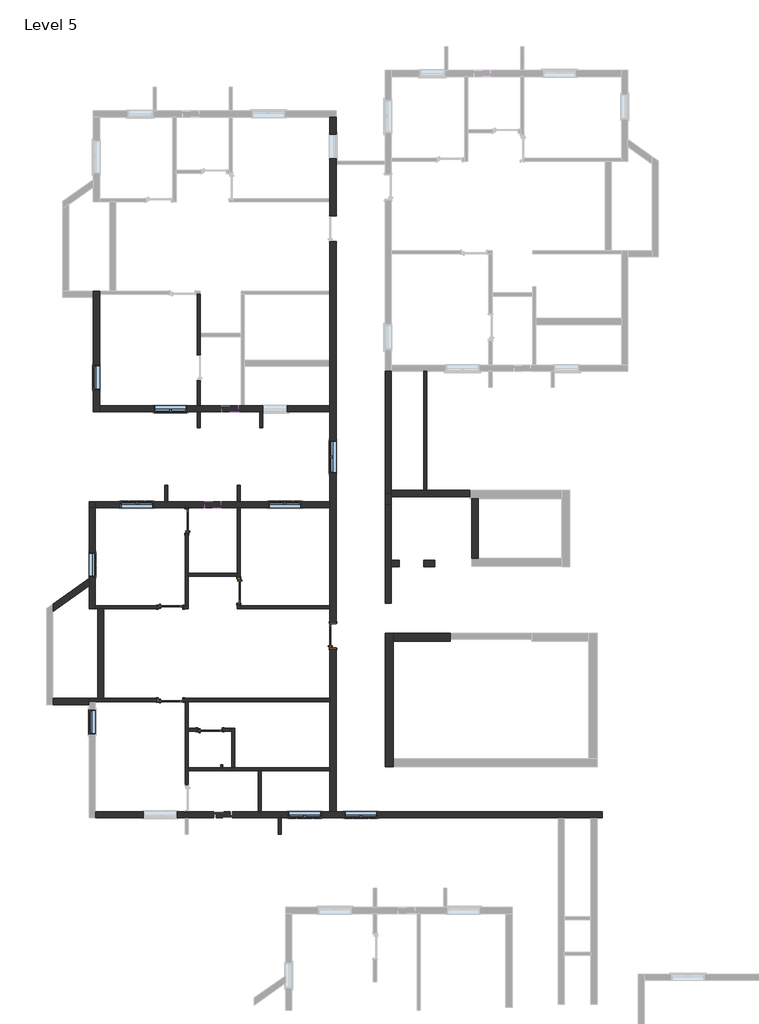
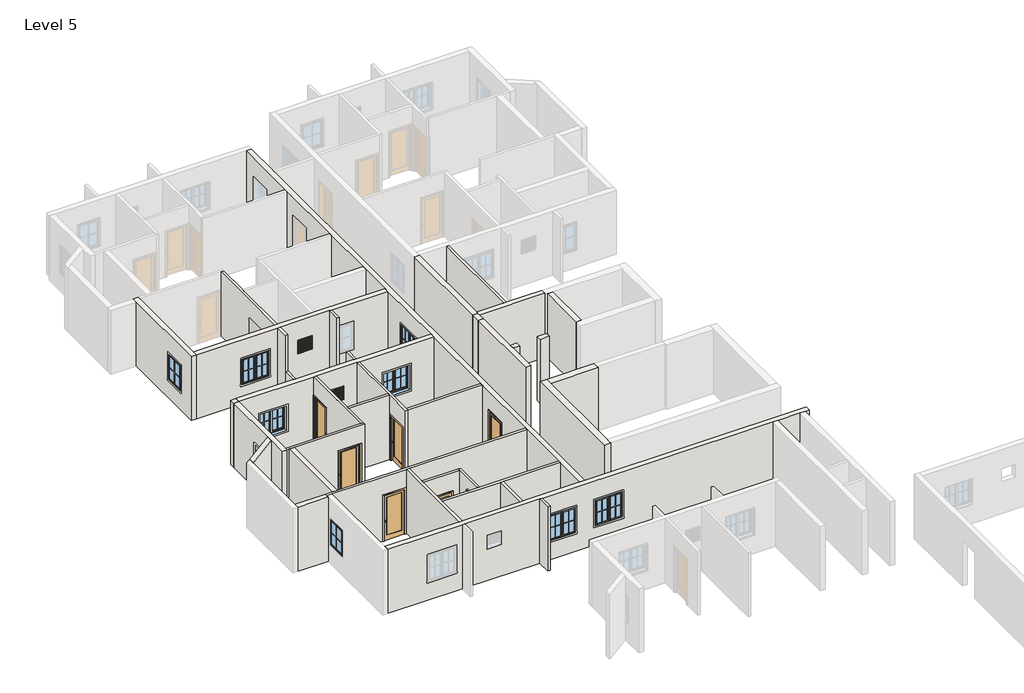
# One storey, part 4 of 7: 38 walls, 11 windows, 6 doors.
"""IFC4 building model written with IfcOpenShell, lengths in millimetres."""

from ifc_helpers import new_model, si_unit, frame, origin, place, context, project, spatial, polyline, outline, extrude, faceted_brep, transform, mapped, element, save
from components import door_a3feeac7, door_3c6ab76a, door_3b97b8e7, window_272f20d6, window_casement_double_4_x_4_af3140d2, window_f2d8fef0

model = new_model("IFC4")

# Units and contexts
model_context = context("Model", 3, world=origin())
ifc_project = project(units=[si_unit("LENGTHUNIT", "METRE", prefix="MILLI")], contexts=[model_context])

# Site, building, storey
site = spatial("IfcSite", under=ifc_project)
building = spatial("IfcBuilding", under=site)
storey = spatial("IfcBuildingStorey", under=building, Name="Level 5", Elevation=6400.8)

# Doors
placement = place(None, origin())
door_shape = door_a3feeac7(model_context)
element("IfcDoor", 1, ObjectType="Door-Interior-Single-1_Panel-Wood : 2'6\" x 7' door", at=placement, inside=storey, context=model_context, shape_type="MappedRepresentation", body=[
    mapped(door_shape, transform((-11252.4759469, 12427.2461172, 6400.8), x_axis=(0.0, 1.0, 0.0), y_axis=(-1.0, 0.0, 0.0), z_axis=(0.0, 0.0, 1.0))),
])
element("IfcDoor", 2, ObjectType="Door-Interior-Single-1_Panel-Wood : 2'6\" x 7' door", at=placement, inside=storey, context=model_context, shape_type="MappedRepresentation", body=[
    mapped(door_shape, transform((-10385.7009469, 4632.6211172, 6400.8), x_axis=(1.0, 0.0, 0.0), y_axis=(0.0, 1.0, 0.0), z_axis=(0.0, 0.0, 1.0))),
])
door_2_shape = door_3c6ab76a(model_context)
element("IfcDoor", 3, ObjectType="Door-Interior-Single-1_Panel-Wood : 36\" x 84\"", at=placement, inside=storey, context=model_context, shape_type="MappedRepresentation", body=[
    mapped(door_2_shape, transform((-9309.3759469, 9817.3961172, 6400.8), x_axis=(0.0, -1.0, 0.0), y_axis=(1.0, 0.0, 0.0), z_axis=(0.0, 0.0, 1.0))),
])
element("IfcDoor", 4, ObjectType="Door-Interior-Single-1_Panel-Wood : 36\" x 84\"", at=placement, inside=storey, context=model_context, shape_type="MappedRepresentation", body=[
    mapped(door_2_shape, transform((-11865.2509469, 9210.9711172, 6400.8), x_axis=(1.0, 0.0, 0.0), y_axis=(0.0, 1.0, 0.0), z_axis=(0.0, 0.0, 1.0))),
])
door_3_shape = door_3b97b8e7(model_context)
element("IfcDoor", 5, ObjectType="Door-Interior-Single-1_Panel-Wood : 36\" x 84\"", at=placement, inside=storey, context=model_context, shape_type="MappedRepresentation", body=[
    mapped(door_3_shape, transform((-5791.4759469, 8140.9961172, 6400.8), x_axis=(0.0, 1.0, 0.0), y_axis=(-1.0, 0.0, 0.0), z_axis=(0.0, 0.0, 1.0))),
])
element("IfcDoor", 6, ObjectType="Door-Interior-Single-1_Panel-Wood : 36\" x 84\"", at=placement, inside=storey, context=model_context, shape_type="MappedRepresentation", body=[
    mapped(door_shape, transform((-11865.2509469, 5737.5211172, 6400.8), x_axis=(1.0, 0.0, 0.0), y_axis=(0.0, 1.0, 0.0), z_axis=(0.0, 0.0, 1.0))),
])

# Walls
element("IfcWall", 7, ObjectType="1' feet", at=placement, inside=storey, context=model_context, shape_type="Brep", body=[
    faceted_brep([(-3540.4009469, 3245.1461172, 6400.8), (-3540.4009469, 3549.9461172, 6400.8), (-3540.4009469, 7931.4461172, 6400.8), (-3540.4009469, 8236.2461172, 6400.8), (-3540.4009469, 8236.2461172, 9448.8), (-3540.4009469, 7931.4461172, 9448.8), (-3540.4009469, 3549.9461172, 9448.8), (-3540.4009469, 3245.1461172, 9448.8), (-3845.2009469, 3245.1461172, 6400.8), (-3845.2009469, 3245.1461172, 9448.8), (-3845.2009469, 8236.2461172, 9448.8), (-3845.2009469, 8236.2461172, 6400.8)], [[[0, 1, 2, 3, 4, 5, 6, 7]], [[8, 9, 10, 11]], [[3, 2, 1, 0, 8, 11]], [[7, 6, 5, 4, 10, 9]], [[4, 3, 11, 10]], [[0, 7, 9, 8]]]),
])
element("IfcWall", 8, ObjectType="1' feet", at=placement, inside=storey, context=model_context, shape_type="Brep", body=[
    faceted_brep([(-3540.4009469, 7931.4461172, 6400.8), (-1406.8009469, 7931.4461172, 6400.8), (-1406.8009469, 7931.4461172, 9448.8), (-3540.4009469, 7931.4461172, 9448.8), (-3540.4009469, 8236.2461172, 6400.8), (-3540.4009469, 8236.2461172, 9448.8), (-1406.8009469, 8236.2461172, 9448.8), (-1406.8009469, 8236.2461172, 6400.8), (-1406.8009469, 8007.6461172, 6400.8), (-1406.8009469, 8007.6461172, 9448.8)], [[[0, 1, 2, 3]], [[4, 5, 6, 7]], [[1, 0, 4, 7, 8]], [[2, 1, 8, 7, 6, 9]], [[3, 2, 9, 6, 5]], [[0, 3, 5, 4]]]),
])
element("IfcWall", 9, ObjectType="4.5\" wall", at=placement, inside=storey, context=model_context, shape_type="Brep", body=[
    faceted_brep([(-10741.3009469, 20898.1461172, 9448.8), (-10741.3009469, 19437.6461172, 9448.8), (-10741.3009469, 19323.3461172, 9448.8), (-10741.3009469, 16732.5461172, 9448.8), (-10741.3009469, 16732.5461172, 6400.8), (-10741.3009469, 17678.6961172, 6400.8), (-10741.3009469, 17678.6961172, 8559.8), (-10741.3009469, 18643.8961172, 8559.8), (-10741.3009469, 18643.8961172, 6400.8), (-10741.3009469, 19323.3461172, 6400.8), (-10741.3009469, 19437.6461172, 6400.8), (-10741.3009469, 20898.1461172, 6400.8), (-10855.6009469, 16732.5461172, 9448.8), (-10855.6009469, 20898.1461172, 9448.8), (-10855.6009469, 20898.1461172, 6400.8), (-10855.6009469, 18643.8961172, 6400.8), (-10855.6009469, 18643.8961172, 8559.8), (-10855.6009469, 17678.6961172, 8559.8), (-10855.6009469, 17678.6961172, 6400.8), (-10855.6009469, 16732.5461172, 6400.8)], [[[0, 1, 2, 3, 4, 5, 6, 7, 8, 9, 10, 11]], [[12, 13, 14, 15, 16, 17, 18, 19]], [[4, 19, 18, 5]], [[14, 11, 10, 9, 8, 15]], [[3, 2, 1, 0, 13, 12]], [[4, 3, 12, 19]], [[0, 11, 14, 13]], [[7, 16, 15, 8]], [[16, 7, 6, 17]], [[17, 6, 5, 18]]]),
])
element("IfcWall", 10, ObjectType="4.5\" wall", at=placement, inside=storey, context=model_context, shape_type="Brep", body=[
    faceted_brep([(-9369.7009469, 9150.6461172, 9448.8), (-9369.7009469, 10369.8461172, 9448.8), (-9369.7009469, 10484.1461172, 9448.8), (-9369.7009469, 12922.5461172, 9448.8), (-9369.7009469, 12922.5461172, 6400.8), (-9369.7009469, 10484.1461172, 6400.8), (-9369.7009469, 10369.8461172, 6400.8), (-9369.7009469, 10299.9961172, 6400.8), (-9369.7009469, 10299.9961172, 8559.8), (-9369.7009469, 9334.7961172, 8559.8), (-9369.7009469, 9334.7961172, 6400.8), (-9369.7009469, 9150.6461172, 6400.8), (-9255.4009469, 12922.5461172, 9448.8), (-9255.4009469, 9264.9461172, 9448.8), (-9255.4009469, 9150.6461172, 9448.8), (-9255.4009469, 9150.6461172, 6400.8), (-9255.4009469, 9264.9461172, 6400.8), (-9255.4009469, 9334.7961172, 6400.8), (-9255.4009469, 9334.7961172, 8559.8), (-9255.4009469, 10299.9961172, 8559.8), (-9255.4009469, 10299.9961172, 6400.8), (-9255.4009469, 12922.5461172, 6400.8)], [[[0, 1, 2, 3, 4, 5, 6, 7, 8, 9, 10, 11]], [[12, 13, 14, 15, 16, 17, 18, 19, 20, 21]], [[4, 21, 20, 7, 6, 5]], [[15, 11, 10, 17, 16]], [[3, 2, 1, 0, 14, 13, 12]], [[4, 3, 12, 21]], [[0, 11, 15, 14]], [[9, 18, 17, 10]], [[18, 9, 8, 19]], [[19, 8, 7, 20]]]),
])
element("IfcWall", 11, ObjectType="4.5\" wall", at=placement, inside=storey, context=model_context, shape_type="SweptSolid", body=[
    extrude(outline(polyline([(-11198.5009469, 10484.1461172), (-9369.7009469, 10484.1461172), (-9369.7009469, 10369.8461172), (-11198.5009469, 10369.8461172), (-11198.5009469, 10484.1461172)])), frame((0.0, 0.0, 6400.8), z_axis=(0.0, 0.0, 1.0), x_axis=(1.0, 0.0, 0.0)), (0.0, 0.0, 1.0), 3048.0),
])
element("IfcWall", 12, ObjectType="4.5\" wall", at=placement, inside=storey, context=model_context, shape_type="Brep", body=[
    faceted_brep([(-11312.8009469, 9264.9461172, 9448.8), (-11312.8009469, 12922.5461172, 9448.8), (-11312.8009469, 12922.5461172, 6400.8), (-11312.8009469, 12909.8461172, 6400.8), (-11312.8009469, 12909.8461172, 8559.8), (-11312.8009469, 11944.6461172, 8559.8), (-11312.8009469, 11944.6461172, 6400.8), (-11312.8009469, 9264.9461172, 6400.8), (-11198.5009469, 12922.5461172, 9448.8), (-11198.5009469, 10484.1461172, 9448.8), (-11198.5009469, 10369.8461172, 9448.8), (-11198.5009469, 9264.9461172, 9448.8), (-11198.5009469, 9264.9461172, 6400.8), (-11198.5009469, 10369.8461172, 6400.8), (-11198.5009469, 10484.1461172, 6400.8), (-11198.5009469, 11944.6461172, 6400.8), (-11198.5009469, 11944.6461172, 8559.8), (-11198.5009469, 12909.8461172, 8559.8), (-11198.5009469, 12909.8461172, 6400.8), (-11198.5009469, 12922.5461172, 6400.8)], [[[0, 1, 2, 3, 4, 5, 6, 7]], [[8, 9, 10, 11, 12, 13, 14, 15, 16, 17, 18, 19]], [[12, 7, 6, 15, 14, 13]], [[2, 19, 18, 3]], [[1, 0, 11, 10, 9, 8]], [[0, 7, 12, 11]], [[2, 1, 8, 19]], [[17, 4, 3, 18]], [[4, 17, 16, 5]], [[5, 16, 15, 6]]]),
])
element("IfcWall", 13, ObjectType="4.5\" wall", at=placement, inside=storey, context=model_context, shape_type="Brep", body=[
    faceted_brep([(-14665.6009469, 9264.9461172, 9448.8), (-11312.8009469, 9264.9461172, 9448.8), (-11198.5009469, 9264.9461172, 9448.8), (-11198.5009469, 9264.9461172, 6400.8), (-11312.8009469, 9264.9461172, 6400.8), (-11382.6509469, 9264.9461172, 6400.8), (-11382.6509469, 9264.9461172, 8559.8), (-12347.8509469, 9264.9461172, 8559.8), (-12347.8509469, 9264.9461172, 6400.8), (-14665.6009469, 9264.9461172, 6400.8), (-11198.5009469, 9150.6461172, 9448.8), (-14360.8009469, 9150.6461172, 9448.8), (-14589.4009469, 9150.6461172, 9448.8), (-14665.6009469, 9150.6461172, 9448.8), (-14665.6009469, 9150.6461172, 6400.8), (-14589.4009469, 9150.6461172, 6400.8), (-14360.8009469, 9150.6461172, 6400.8), (-12347.8509469, 9150.6461172, 6400.8), (-12347.8509469, 9150.6461172, 8559.8), (-11382.6509469, 9150.6461172, 8559.8), (-11382.6509469, 9150.6461172, 6400.8), (-11198.5009469, 9150.6461172, 6400.8)], [[[0, 1, 2, 3, 4, 5, 6, 7, 8, 9]], [[10, 11, 12, 13, 14, 15, 16, 17, 18, 19, 20, 21]], [[3, 21, 20, 5, 4]], [[14, 9, 8, 17, 16, 15]], [[2, 1, 0, 13, 12, 11, 10]], [[3, 2, 10, 21]], [[0, 9, 14, 13]], [[19, 6, 5, 20]], [[6, 19, 18, 7]], [[7, 18, 17, 8]]]),
])
element("IfcWall", 14, ObjectType="4.5\" wall", at=placement, inside=storey, context=model_context, shape_type="SweptSolid", body=[
    extrude(outline(polyline([(-9255.4009469, 9264.9461172), (-5902.6009469, 9264.9461172), (-5902.6009469, 9150.6461172), (-9255.4009469, 9150.6461172), (-9255.4009469, 9264.9461172)])), frame((0.0, 0.0, 6400.8), z_axis=(0.0, 0.0, 1.0), x_axis=(1.0, 0.0, 0.0)), (0.0, 0.0, 1.0), 3048.0),
])
element("IfcWall", 15, ObjectType="4.5\" wall", at=placement, inside=storey, context=model_context, shape_type="Brep", body=[
    faceted_brep([(-5902.6009469, 5683.5461172, 9448.8), (-11198.5009469, 5683.5461172, 9448.8), (-11312.8009469, 5683.5461172, 9448.8), (-14665.6009469, 5683.5461172, 9448.8), (-14894.2009469, 5683.5461172, 9448.8), (-14894.2009469, 5683.5461172, 6400.8), (-14665.6009469, 5683.5461172, 6400.8), (-12347.8509469, 5683.5461172, 6400.8), (-12347.8509469, 5683.5461172, 8559.8), (-11382.6509469, 5683.5461172, 8559.8), (-11382.6509469, 5683.5461172, 6400.8), (-11312.8009469, 5683.5461172, 6400.8), (-11198.5009469, 5683.5461172, 6400.8), (-5902.6009469, 5683.5461172, 6400.8), (-14894.2009469, 5797.8461172, 9448.8), (-14589.4009469, 5797.8461172, 9448.8), (-14360.8009469, 5797.8461172, 9448.8), (-5902.6009469, 5797.8461172, 9448.8), (-5902.6009469, 5797.8461172, 6400.8), (-11382.6509469, 5797.8461172, 6400.8), (-11382.6509469, 5797.8461172, 8559.8), (-12347.8509469, 5797.8461172, 8559.8), (-12347.8509469, 5797.8461172, 6400.8), (-14360.8009469, 5797.8461172, 6400.8), (-14589.4009469, 5797.8461172, 6400.8), (-14894.2009469, 5797.8461172, 6400.8)], [[[0, 1, 2, 3, 4, 5, 6, 7, 8, 9, 10, 11, 12, 13]], [[14, 15, 16, 17, 18, 19, 20, 21, 22, 23, 24, 25]], [[18, 13, 12, 11, 10, 19]], [[5, 25, 24, 23, 22, 7, 6]], [[4, 3, 2, 1, 0, 17, 16, 15, 14]], [[0, 13, 18, 17]], [[5, 4, 14, 25]], [[9, 20, 19, 10]], [[20, 9, 8, 21]], [[21, 8, 7, 22]]]),
])
element("IfcWall", 16, ObjectType="4.5\" wall", at=placement, inside=storey, context=model_context, shape_type="Brep", body=[
    faceted_brep([(-11198.5009469, 5683.5461172, 9448.8), (-11198.5009469, 4692.9461172, 9448.8), (-11198.5009469, 4578.6461172, 9448.8), (-11198.5009469, 3207.0461172, 9448.8), (-11198.5009469, 3092.7461172, 9448.8), (-11198.5009469, 1568.7461172, 9448.8), (-11198.5009469, 1568.7461172, 6400.8), (-11198.5009469, 1581.4461172, 6400.8), (-11198.5009469, 1581.4461172, 8559.8), (-11198.5009469, 2546.6461172, 8559.8), (-11198.5009469, 2546.6461172, 6400.8), (-11198.5009469, 3092.7461172, 6400.8), (-11198.5009469, 3207.0461172, 6400.8), (-11198.5009469, 4578.6461172, 6400.8), (-11198.5009469, 4692.9461172, 6400.8), (-11198.5009469, 5683.5461172, 6400.8), (-11312.8009469, 1568.7461172, 9448.8), (-11312.8009469, 5683.5461172, 9448.8), (-11312.8009469, 5683.5461172, 6400.8), (-11312.8009469, 2546.6461172, 6400.8), (-11312.8009469, 2546.6461172, 8559.8), (-11312.8009469, 1581.4461172, 8559.8), (-11312.8009469, 1581.4461172, 6400.8), (-11312.8009469, 1568.7461172, 6400.8)], [[[0, 1, 2, 3, 4, 5, 6, 7, 8, 9, 10, 11, 12, 13, 14, 15]], [[16, 17, 18, 19, 20, 21, 22, 23]], [[18, 15, 14, 13, 12, 11, 10, 19]], [[6, 23, 22, 7]], [[5, 4, 3, 2, 1, 0, 17, 16]], [[0, 15, 18, 17]], [[6, 5, 16, 23]], [[21, 8, 7, 22]], [[8, 21, 20, 9]], [[9, 20, 19, 10]]]),
])
element("IfcWall", 17, ObjectType="4.5\" wall", at=placement, inside=storey, context=model_context, shape_type="SweptSolid", body=[
    extrude(outline(polyline([(-9985.226836, 3326.5226372), (-9915.376836, 3326.5226372), (-9915.376836, 3212.2226372), (-9985.226836, 3212.2226372), (-9985.226836, 3326.5226372)])), frame((0.0, 0.0, 6400.8), z_axis=(0.0, 0.0, 1.0), x_axis=(1.0, 0.0, 0.0)), (0.0, 0.0, 1.0), 3048.0),
])
element("IfcWall", 18, ObjectType="4.5\" wall", at=placement, inside=storey, context=model_context, shape_type="Brep", body=[
    faceted_brep([(-5902.6009469, 3207.0461172, 6400.8), (-11198.5009469, 3207.0461172, 6400.8), (-11198.5009469, 3207.0461172, 9448.8), (-5902.6009469, 3207.0461172, 9448.8), (-5902.6009469, 3092.7461172, 6400.8), (-5902.6009469, 3092.7461172, 9448.8), (-8468.0009469, 3092.7461172, 9448.8), (-8582.3009469, 3092.7461172, 9448.8), (-11198.5009469, 3092.7461172, 9448.8), (-11198.5009469, 3092.7461172, 6400.8), (-8582.3009469, 3092.7461172, 6400.8), (-8468.0009469, 3092.7461172, 6400.8)], [[[0, 1, 2, 3]], [[4, 5, 6, 7, 8, 9, 10, 11]], [[1, 0, 4, 11, 10, 9]], [[3, 2, 8, 7, 6, 5]], [[2, 1, 9, 8]], [[0, 3, 5, 4]]]),
])
element("IfcWall", 19, ObjectType="4.5\" wall", at=placement, inside=storey, context=model_context, shape_type="SweptSolid", body=[
    extrude(outline(polyline([(-8582.3009469, 1568.7461172), (-8582.3009469, 3092.7461172), (-8468.0009469, 3092.7461172), (-8468.0009469, 1568.7461172), (-8582.3009469, 1568.7461172)])), frame((0.0, 0.0, 6400.8), z_axis=(0.0, 0.0, 1.0), x_axis=(1.0, 0.0, 0.0)), (0.0, 0.0, 1.0), 3048.0),
])
element("IfcWall", 20, ObjectType="4.5\" wall", at=placement, inside=storey, context=model_context, shape_type="Brep", body=[
    faceted_brep([(-9572.9009469, 4692.9461172, 6400.8), (-9572.9009469, 4578.6461172, 6400.8), (-9572.9009469, 3245.1461172, 6400.8), (-9572.9009469, 3245.1461172, 9448.8), (-9572.9009469, 4578.6461172, 9448.8), (-9572.9009469, 4692.9461172, 9448.8), (-9458.6009469, 4692.9461172, 6400.8), (-9458.6009469, 4692.9461172, 9448.8), (-9458.6009469, 3245.1461172, 9448.8), (-9458.6009469, 3245.1461172, 6400.8)], [[[0, 1, 2, 3, 4, 5]], [[6, 7, 8, 9]], [[2, 1, 0, 6, 9]], [[3, 2, 9, 8]], [[5, 4, 3, 8, 7]], [[0, 5, 7, 6]]]),
])
element("IfcWall", 21, ObjectType="4.5\" wall", at=placement, inside=storey, context=model_context, shape_type="SweptSolid", body=[
    extrude(outline(polyline([(9448.8, -9572.9009469), (9448.8, -11198.5009469), (6400.8, -11198.5009469), (6400.8, -10868.3009469), (8559.8, -10868.3009469), (8559.8, -9903.1009469), (6400.8, -9903.1009469), (6400.8, -9572.9009469), (9448.8, -9572.9009469)])), frame((0.0, 4578.6461172, 0.0), z_axis=(0.0, 1.0, 0.0), x_axis=(0.0, 0.0, 1.0)), (0.0, 0.0, 1.0), 114.3),
])
element("IfcWall", 22, ObjectType="4.5\" wall", at=placement, inside=storey, context=model_context, shape_type="SweptSolid", body=[
    extrude(outline(polyline([(-7841.0333092, 730.5461172), (-7841.0333092, 1340.1461172), (-7726.7333092, 1340.1461172), (-7726.7333092, 730.5461172), (-7841.0333092, 730.5461172)])), frame((0.0, 0.0, 6400.8), z_axis=(0.0, 0.0, 1.0), x_axis=(1.0, 0.0, 0.0)), (0.0, 0.0, 1.0), 3048.0),
])
element("IfcWall", 23, ObjectType="4.5\" wall", at=placement, inside=storey, context=model_context, shape_type="SweptSolid", body=[
    extrude(outline(polyline([(-10855.6009469, 15918.3895495), (-10855.6009469, 16503.9461172), (-10741.3009469, 16503.9461172), (-10741.3009469, 15918.3895495), (-10855.6009469, 15918.3895495)])), frame((0.0, 0.0, 6400.8), z_axis=(0.0, 0.0, 1.0), x_axis=(1.0, 0.0, 0.0)), (0.0, 0.0, 1.0), 3048.0),
])
element("IfcWall", 24, ObjectType="4.5\" wall", at=placement, inside=storey, context=model_context, shape_type="Brep", body=[
    faceted_brep([(-8531.5009469, 16503.9461172, 6400.8), (-8531.5009469, 15918.3895495, 6400.8), (-8531.5009469, 15918.3895495, 9448.8), (-8531.5009469, 16503.9461172, 9448.8), (-8417.2009469, 16503.9461172, 6400.8), (-8417.2009469, 16503.9461172, 7315.2), (-8417.2009469, 16503.9461172, 8534.4), (-8417.2009469, 16503.9461172, 9448.8), (-8417.2009469, 15918.3895495, 9448.8), (-8417.2009469, 15918.3895495, 6400.8)], [[[0, 1, 2, 3]], [[4, 5, 6, 7, 8, 9]], [[1, 0, 4, 9]], [[2, 1, 9, 8]], [[3, 2, 8, 7]], [[0, 3, 7, 6, 5, 4]]]),
])
element("IfcWall", 25, ObjectType="4.5\" wall", at=placement, inside=storey, context=model_context, shape_type="SweptSolid", body=[
    extrude(outline(polyline([(-12085.9698258, 13151.1461172), (-12085.9698258, 13760.7461172), (-11971.6698258, 13760.7461172), (-11971.6698258, 13151.1461172), (-12085.9698258, 13151.1461172)])), frame((0.0, 0.0, 6400.8), z_axis=(0.0, 0.0, 1.0), x_axis=(1.0, 0.0, 0.0)), (0.0, 0.0, 1.0), 3048.0),
])
element("IfcWall", 26, ObjectType="4.5\" wall", at=placement, inside=storey, context=model_context, shape_type="SweptSolid", body=[
    extrude(outline(polyline([(-9255.4009469, 13760.7461172), (-9255.4009469, 13151.1461172), (-9369.7009469, 13151.1461172), (-9369.7009469, 13760.7461172), (-9255.4009469, 13760.7461172)])), frame((0.0, 0.0, 6400.8), z_axis=(0.0, 0.0, 1.0), x_axis=(1.0, 0.0, 0.0)), (0.0, 0.0, 1.0), 3048.0),
])
element("IfcWall", 27, ObjectType="4.5\" wall", at=placement, inside=storey, context=model_context, shape_type="SweptSolid", body=[
    extrude(outline(polyline([(-2402.381873, 13571.4182723), (-2402.381873, 18017.4255084), (-2288.081873, 18017.4255084), (-2288.081873, 13571.4182723), (-2402.381873, 13571.4182723)])), frame((0.0, 0.0, 6400.8), z_axis=(0.0, 0.0, 1.0), x_axis=(1.0, 0.0, 0.0)), (0.0, 0.0, 1.0), 3048.0),
])
element("IfcWall", 28, ObjectType="9\"", at=placement, inside=storey, context=model_context, shape_type="Brep", body=[
    faceted_brep([(-14513.2009469, 16503.9461172, 6400.8), (-14513.2009469, 16732.5461172, 6400.8), (-14513.2009469, 20898.1461172, 6400.8), (-14513.2009469, 21012.4461172, 6400.8), (-14513.2009469, 21012.4461172, 9448.8), (-14513.2009469, 20898.1461172, 9448.8), (-14513.2009469, 16732.5461172, 9448.8), (-14513.2009469, 16503.9461172, 9448.8), (-14513.2009469, 18243.8461172, 8534.4), (-14513.2009469, 18243.8461172, 7315.2), (-14513.2009469, 17329.4461172, 7315.2), (-14513.2009469, 17329.4461172, 8534.4), (-14741.8009469, 16503.9461172, 6400.8), (-14741.8009469, 16503.9461172, 9448.8), (-14741.8009469, 20783.8461172, 9448.8), (-14741.8009469, 21012.4461172, 9448.8), (-14741.8009469, 21012.4461172, 6400.8), (-14741.8009469, 20783.8461172, 6400.8), (-14741.8009469, 18243.8461172, 8534.4), (-14741.8009469, 17329.4461172, 8534.4), (-14741.8009469, 17329.4461172, 7315.2), (-14741.8009469, 18243.8461172, 7315.2)], [[[0, 1, 2, 3, 4, 5, 6, 7], [8, 9, 10, 11]], [[12, 13, 14, 15, 16, 17], [18, 19, 20, 21]], [[3, 2, 1, 0, 12, 17, 16]], [[7, 6, 5, 4, 15, 14, 13]], [[4, 3, 16, 15]], [[0, 7, 13, 12]], [[9, 8, 18, 21]], [[10, 9, 21, 20]], [[11, 10, 20, 19]], [[8, 11, 19, 18]]]),
])
element("IfcWall", 29, ObjectType="9\"", at=placement, inside=storey, context=model_context, shape_type="Brep", body=[
    faceted_brep([(-5902.6009469, 1568.7461172, 9448.8), (-5902.6009469, 3092.7461172, 9448.8), (-5902.6009469, 3207.0461172, 9448.8), (-5902.6009469, 5683.5461172, 9448.8), (-5902.6009469, 5797.8461172, 9448.8), (-5902.6009469, 9150.6461172, 9448.8), (-5902.6009469, 9264.9461172, 9448.8), (-5902.6009469, 12922.5461172, 9448.8), (-5902.6009469, 13151.1461172, 9448.8), (-5902.6009469, 16503.9461172, 9448.8), (-5902.6009469, 16732.5461172, 9448.8), (-5902.6009469, 18205.7461172, 9448.8), (-5902.6009469, 18434.3461172, 9448.8), (-5902.6009469, 20898.1461172, 9448.8), (-5902.6009469, 21012.4461172, 9448.8), (-5902.6009469, 24365.2461172, 9448.8), (-5902.6009469, 24479.5461172, 9448.8), (-5902.6009469, 27527.5461172, 9448.8), (-5902.6009469, 27527.5461172, 6400.8), (-5902.6009469, 24479.5461172, 6400.8), (-5902.6009469, 24365.2461172, 6400.8), (-5902.6009469, 23838.1961172, 6400.8), (-5902.6009469, 23838.1961172, 8559.8), (-5902.6009469, 22872.9961172, 8559.8), (-5902.6009469, 22872.9961172, 6400.8), (-5902.6009469, 21012.4461172, 6400.8), (-5902.6009469, 20898.1461172, 6400.8), (-5902.6009469, 18434.3461172, 6400.8), (-5902.6009469, 18205.7461172, 6400.8), (-5902.6009469, 16732.5461172, 6400.8), (-5902.6009469, 16503.9461172, 6400.8), (-5902.6009469, 13151.1461172, 6400.8), (-5902.6009469, 12922.5461172, 6400.8), (-5902.6009469, 9264.9461172, 6400.8), (-5902.6009469, 9150.6461172, 6400.8), (-5902.6009469, 8623.5961172, 6400.8), (-5902.6009469, 8623.5961172, 8559.8), (-5902.6009469, 7658.3961172, 8559.8), (-5902.6009469, 7658.3961172, 6400.8), (-5902.6009469, 5797.8461172, 6400.8), (-5902.6009469, 5683.5461172, 6400.8), (-5902.6009469, 3207.0461172, 6400.8), (-5902.6009469, 3092.7461172, 6400.8), (-5902.6009469, 1568.7461172, 6400.8), (-5902.6009469, 25973.9755084, 8534.4), (-5902.6009469, 25973.9755084, 7315.2), (-5902.6009469, 26888.3755084, 7315.2), (-5902.6009469, 26888.3755084, 8534.4), (-5902.6009469, 15437.1461172, 8534.4), (-5902.6009469, 14217.9461172, 8534.4), (-5902.6009469, 14217.9461172, 7315.2), (-5902.6009469, 15437.1461172, 7315.2), (-5674.0009469, 27527.5461172, 9448.8), (-5674.0009469, 25878.7255084, 9448.8), (-5674.0009469, 25764.4255084, 9448.8), (-5674.0009469, 1568.7461172, 9448.8), (-5674.0009469, 1568.7461172, 6400.8), (-5674.0009469, 7658.3961172, 6400.8), (-5674.0009469, 7658.3961172, 8559.8), (-5674.0009469, 8623.5961172, 8559.8), (-5674.0009469, 8623.5961172, 6400.8), (-5674.0009469, 22872.9961172, 6400.8), (-5674.0009469, 22872.9961172, 8559.8), (-5674.0009469, 23838.1961172, 8559.8), (-5674.0009469, 23838.1961172, 6400.8), (-5674.0009469, 25764.4255084, 6400.8), (-5674.0009469, 25878.7255084, 6400.8), (-5674.0009469, 27527.5461172, 6400.8), (-5674.0009469, 27527.5461172, 6553.2), (-5674.0009469, 25973.9755084, 8534.4), (-5674.0009469, 26888.3755084, 8534.4), (-5674.0009469, 26888.3755084, 7315.2), (-5674.0009469, 25973.9755084, 7315.2), (-5674.0009469, 15437.1461172, 8534.4), (-5674.0009469, 15437.1461172, 7315.2), (-5674.0009469, 14217.9461172, 7315.2), (-5674.0009469, 14217.9461172, 8534.4)], [[[0, 1, 2, 3, 4, 5, 6, 7, 8, 9, 10, 11, 12, 13, 14, 15, 16, 17, 18, 19, 20, 21, 22, 23, 24, 25, 26, 27, 28, 29, 30, 31, 32, 33, 34, 35, 36, 37, 38, 39, 40, 41, 42, 43], [44, 45, 46, 47], [48, 49, 50, 51]], [[52, 53, 54, 55, 56, 57, 58, 59, 60, 61, 62, 63, 64, 65, 66, 67, 68], [69, 70, 71, 72], [73, 74, 75, 76]], [[18, 67, 66, 65, 64, 21, 20, 19]], [[56, 43, 42, 41, 40, 39, 38, 57]], [[24, 61, 60, 35, 34, 33, 32, 31, 30, 29, 28, 27, 26, 25]], [[17, 16, 15, 14, 13, 12, 11, 10, 9, 8, 7, 6, 5, 4, 3, 2, 1, 0, 55, 54, 53, 52]], [[18, 17, 52, 68, 67]], [[0, 43, 56, 55]], [[63, 22, 21, 64]], [[22, 63, 62, 23]], [[23, 62, 61, 24]], [[59, 36, 35, 60]], [[36, 59, 58, 37]], [[37, 58, 57, 38]], [[45, 44, 69, 72]], [[46, 45, 72, 71]], [[47, 46, 71, 70]], [[44, 47, 70, 69]], [[74, 73, 48, 51]], [[75, 74, 51, 50]], [[76, 75, 50, 49]], [[73, 76, 49, 48]]]),
])
element("IfcWall", 30, ObjectType="9\"", at=placement, inside=storey, context=model_context, shape_type="Brep", body=[
    faceted_brep([(-14513.2009469, 16503.9461172, 6400.8), (-10855.6009469, 16503.9461172, 6400.8), (-10741.3009469, 16503.9461172, 6400.8), (-8531.5009469, 16503.9461172, 6400.8), (-8417.2009469, 16503.9461172, 6400.8), (-5902.6009469, 16503.9461172, 6400.8), (-5902.6009469, 16503.9461172, 9448.8), (-8417.2009469, 16503.9461172, 9448.8), (-8531.5009469, 16503.9461172, 9448.8), (-10741.3009469, 16503.9461172, 9448.8), (-10855.6009469, 16503.9461172, 9448.8), (-14513.2009469, 16503.9461172, 9448.8), (-9337.9509469, 16503.9461172, 8534.4), (-9337.9509469, 16503.9461172, 7924.8), (-9947.5509469, 16503.9461172, 7924.8), (-9947.5509469, 16503.9461172, 8534.4), (-8417.2009469, 16503.9461172, 8534.4), (-7502.8009469, 16503.9461172, 8534.4), (-7502.8009469, 16503.9461172, 7315.2), (-8417.2009469, 16503.9461172, 7315.2), (-12474.8509469, 16503.9461172, 8534.4), (-11255.6509469, 16503.9461172, 8534.4), (-11255.6509469, 16503.9461172, 7315.2), (-12474.8509469, 16503.9461172, 7315.2), (-14513.2009469, 16732.5461172, 6400.8), (-14513.2009469, 16732.5461172, 9448.8), (-10855.6009469, 16732.5461172, 9448.8), (-10741.3009469, 16732.5461172, 9448.8), (-9217.3009469, 16732.5461172, 9448.8), (-9103.0009469, 16732.5461172, 9448.8), (-5902.6009469, 16732.5461172, 9448.8), (-5902.6009469, 16732.5461172, 6400.8), (-9103.0009469, 16732.5461172, 6400.8), (-9217.3009469, 16732.5461172, 6400.8), (-10741.3009469, 16732.5461172, 6400.8), (-10855.6009469, 16732.5461172, 6400.8), (-9337.9509469, 16732.5461172, 8534.4), (-9947.5509469, 16732.5461172, 8534.4), (-9947.5509469, 16732.5461172, 7924.8), (-9337.9509469, 16732.5461172, 7924.8), (-8417.2009469, 16732.5461172, 8534.4), (-8417.2009469, 16732.5461172, 7315.2), (-7502.8009469, 16732.5461172, 7315.2), (-7502.8009469, 16732.5461172, 8534.4), (-12474.8509469, 16732.5461172, 8534.4), (-12474.8509469, 16732.5461172, 7315.2), (-11255.6509469, 16732.5461172, 7315.2), (-11255.6509469, 16732.5461172, 8534.4)], [[[0, 1, 2, 3, 4, 5, 6, 7, 8, 9, 10, 11], [12, 13, 14, 15], [16, 17, 18, 19], [20, 21, 22, 23]], [[24, 25, 26, 27, 28, 29, 30, 31, 32, 33, 34, 35], [36, 37, 38, 39], [40, 41, 42, 43], [44, 45, 46, 47]], [[5, 4, 3, 2, 1, 0, 24, 35, 34, 33, 32, 31]], [[11, 10, 9, 8, 7, 6, 30, 29, 28, 27, 26, 25]], [[6, 5, 31, 30]], [[0, 11, 25, 24]], [[13, 12, 36, 39]], [[14, 13, 39, 38]], [[15, 14, 38, 37]], [[12, 15, 37, 36]], [[41, 40, 16, 19]], [[42, 41, 19, 18]], [[43, 42, 18, 17]], [[40, 43, 17, 16]], [[45, 44, 20, 23]], [[46, 45, 23, 22]], [[47, 46, 22, 21]], [[44, 47, 21, 20]]]),
])
element("IfcWall", 31, ObjectType="9\"", at=placement, inside=storey, context=model_context, shape_type="Brep", body=[
    faceted_brep([(-5902.6009469, 13151.1461172, 6400.8), (-9255.4009469, 13151.1461172, 6400.8), (-9369.7009469, 13151.1461172, 6400.8), (-11971.6698258, 13151.1461172, 6400.8), (-12085.9698258, 13151.1461172, 6400.8), (-14665.6009469, 13151.1461172, 6400.8), (-14665.6009469, 13151.1461172, 9448.8), (-12085.9698258, 13151.1461172, 9448.8), (-11971.6698258, 13151.1461172, 9448.8), (-9369.7009469, 13151.1461172, 9448.8), (-9255.4009469, 13151.1461172, 9448.8), (-5902.6009469, 13151.1461172, 9448.8), (-9979.3009469, 13151.1461172, 8534.4), (-10588.9009469, 13151.1461172, 8534.4), (-10588.9009469, 13151.1461172, 7924.8), (-9979.3009469, 13151.1461172, 7924.8), (-12511.4198258, 13151.1461172, 8534.4), (-13730.6198258, 13151.1461172, 8534.4), (-13730.6198258, 13151.1461172, 7315.2), (-12511.4198258, 13151.1461172, 7315.2), (-6975.7509469, 13151.1461172, 8534.4), (-8194.9509469, 13151.1461172, 8534.4), (-8194.9509469, 13151.1461172, 7315.2), (-6975.7509469, 13151.1461172, 7315.2), (-5902.6009469, 12922.5461172, 6400.8), (-5902.6009469, 12922.5461172, 9448.8), (-9255.4009469, 12922.5461172, 9448.8), (-9369.7009469, 12922.5461172, 9448.8), (-11198.5009469, 12922.5461172, 9448.8), (-11312.8009469, 12922.5461172, 9448.8), (-14665.6009469, 12922.5461172, 9448.8), (-14665.6009469, 12922.5461172, 6400.8), (-11312.8009469, 12922.5461172, 6400.8), (-11198.5009469, 12922.5461172, 6400.8), (-9369.7009469, 12922.5461172, 6400.8), (-9255.4009469, 12922.5461172, 6400.8), (-9979.3009469, 12922.5461172, 8534.4), (-9979.3009469, 12922.5461172, 7924.8), (-10588.9009469, 12922.5461172, 7924.8), (-10588.9009469, 12922.5461172, 8534.4), (-12511.4198258, 12922.5461172, 8534.4), (-12511.4198258, 12922.5461172, 7315.2), (-13730.6198258, 12922.5461172, 7315.2), (-13730.6198258, 12922.5461172, 8534.4), (-6975.7509469, 12922.5461172, 8534.4), (-6975.7509469, 12922.5461172, 7315.2), (-8194.9509469, 12922.5461172, 7315.2), (-8194.9509469, 12922.5461172, 8534.4)], [[[0, 1, 2, 3, 4, 5, 6, 7, 8, 9, 10, 11], [12, 13, 14, 15], [16, 17, 18, 19], [20, 21, 22, 23]], [[24, 25, 26, 27, 28, 29, 30, 31, 32, 33, 34, 35], [36, 37, 38, 39], [40, 41, 42, 43], [44, 45, 46, 47]], [[5, 4, 3, 2, 1, 0, 24, 35, 34, 33, 32, 31]], [[11, 10, 9, 8, 7, 6, 30, 29, 28, 27, 26, 25]], [[6, 5, 31, 30]], [[0, 11, 25, 24]], [[37, 36, 12, 15]], [[38, 37, 15, 14]], [[39, 38, 14, 13]], [[36, 39, 13, 12]], [[41, 40, 16, 19]], [[42, 41, 19, 18]], [[43, 42, 18, 17]], [[40, 43, 17, 16]], [[45, 44, 20, 23]], [[46, 45, 23, 22]], [[47, 46, 22, 21]], [[44, 47, 21, 20]]]),
])
element("IfcWall", 32, ObjectType="9\"", at=placement, inside=storey, context=model_context, shape_type="SweptSolid", body=[
    extrude(outline(polyline([(-14894.2009469, 12922.5461172), (-14894.2009469, 13151.1461172), (-14665.6009469, 13151.1461172), (-14665.6009469, 12922.5461172), (-14894.2009469, 12922.5461172)])), frame((0.0, 0.0, 6400.8), z_axis=(0.0, 0.0, 1.0), x_axis=(1.0, 0.0, 0.0)), (0.0, 0.0, 1.0), 3048.0),
])
element("IfcWall", 33, ObjectType="9\"", at=placement, inside=storey, context=model_context, shape_type="SweptSolid", body=[
    extrude(outline(polyline([(-14589.4009469, 5797.8461172), (-14589.4009469, 9150.6461172), (-14360.8009469, 9150.6461172), (-14360.8009469, 5797.8461172), (-14589.4009469, 5797.8461172)])), frame((0.0, 0.0, 6400.8), z_axis=(0.0, 0.0, 1.0), x_axis=(1.0, 0.0, 0.0)), (0.0, 0.0, 1.0), 3048.0),
])
element("IfcWall", 34, ObjectType="9\"", at=placement, inside=storey, context=model_context, shape_type="Brep", body=[
    faceted_brep([(-14665.6009469, 1340.1461172, 6400.8), (-11312.8009469, 1340.1461172, 6400.8), (-11198.5009469, 1340.1461172, 6400.8), (-7841.0333092, 1340.1461172, 6400.8), (-7726.7333092, 1340.1461172, 6400.8), (2631.7990531, 1340.1461172, 6400.8), (2860.3990531, 1340.1461172, 6400.8), (3850.9990531, 1340.1461172, 6400.8), (4079.5990531, 1340.1461172, 6400.8), (4270.0990531, 1340.1461172, 6400.8), (4270.0990531, 1340.1461172, 9448.8), (4079.5990531, 1340.1461172, 9448.8), (3850.9990531, 1340.1461172, 9448.8), (2860.3990531, 1340.1461172, 9448.8), (2631.7990531, 1340.1461172, 9448.8), (-7726.7333092, 1340.1461172, 9448.8), (-7841.0333092, 1340.1461172, 9448.8), (-11198.5009469, 1340.1461172, 9448.8), (-11312.8009469, 1340.1461172, 9448.8), (-14665.6009469, 1340.1461172, 9448.8), (-10195.2009469, 1340.1461172, 8534.4), (-9585.6009469, 1340.1461172, 8534.4), (-9585.6009469, 1340.1461172, 7924.8), (-10195.2009469, 1340.1461172, 7924.8), (-5356.5009469, 1340.1461172, 8534.4), (-4137.3009469, 1340.1461172, 8534.4), (-4137.3009469, 1340.1461172, 7315.2), (-5356.5009469, 1340.1461172, 7315.2), (-7453.6833092, 1340.1461172, 8534.4), (-6234.4833092, 1340.1461172, 8534.4), (-6234.4833092, 1340.1461172, 7315.2), (-7453.6833092, 1340.1461172, 7315.2), (-12855.8509469, 1340.1461172, 8534.4), (-11636.6509469, 1340.1461172, 8534.4), (-11636.6509469, 1340.1461172, 7315.2), (-12855.8509469, 1340.1461172, 7315.2), (-14665.6009469, 1568.7461172, 6400.8), (-14665.6009469, 1568.7461172, 9448.8), (-11312.8009469, 1568.7461172, 9448.8), (-11198.5009469, 1568.7461172, 9448.8), (-8582.3009469, 1568.7461172, 9448.8), (-8468.0009469, 1568.7461172, 9448.8), (-5902.6009469, 1568.7461172, 9448.8), (-5674.0009469, 1568.7461172, 9448.8), (4270.0990531, 1568.7461172, 9448.8), (4270.0990531, 1568.7461172, 6400.8), (-5674.0009469, 1568.7461172, 6400.8), (-5902.6009469, 1568.7461172, 6400.8), (-8468.0009469, 1568.7461172, 6400.8), (-8582.3009469, 1568.7461172, 6400.8), (-11198.5009469, 1568.7461172, 6400.8), (-11312.8009469, 1568.7461172, 6400.8), (-10195.2009469, 1568.7461172, 8534.4), (-10195.2009469, 1568.7461172, 7924.8), (-9585.6009469, 1568.7461172, 7924.8), (-9585.6009469, 1568.7461172, 8534.4), (-5356.5009469, 1568.7461172, 8534.4), (-5356.5009469, 1568.7461172, 7315.2), (-4137.3009469, 1568.7461172, 7315.2), (-4137.3009469, 1568.7461172, 8534.4), (-7453.6833092, 1568.7461172, 8534.4), (-7453.6833092, 1568.7461172, 7315.2), (-6234.4833092, 1568.7461172, 7315.2), (-6234.4833092, 1568.7461172, 8534.4), (-12855.8509469, 1568.7461172, 8534.4), (-12855.8509469, 1568.7461172, 7315.2), (-11636.6509469, 1568.7461172, 7315.2), (-11636.6509469, 1568.7461172, 8534.4)], [[[0, 1, 2, 3, 4, 5, 6, 7, 8, 9, 10, 11, 12, 13, 14, 15, 16, 17, 18, 19], [20, 21, 22, 23], [24, 25, 26, 27], [28, 29, 30, 31], [32, 33, 34, 35]], [[36, 37, 38, 39, 40, 41, 42, 43, 44, 45, 46, 47, 48, 49, 50, 51], [52, 53, 54, 55], [56, 57, 58, 59], [60, 61, 62, 63], [64, 65, 66, 67]], [[9, 8, 7, 6, 5, 4, 3, 2, 1, 0, 36, 51, 50, 49, 48, 47, 46, 45]], [[10, 9, 45, 44]], [[19, 18, 17, 16, 15, 14, 13, 12, 11, 10, 44, 43, 42, 41, 40, 39, 38, 37]], [[0, 19, 37, 36]], [[53, 52, 20, 23]], [[54, 53, 23, 22]], [[55, 54, 22, 21]], [[52, 55, 21, 20]], [[57, 56, 24, 27]], [[58, 57, 27, 26]], [[59, 58, 26, 25]], [[56, 59, 25, 24]], [[61, 60, 28, 31]], [[62, 61, 31, 30]], [[63, 62, 30, 29]], [[60, 63, 29, 28]], [[65, 64, 32, 35]], [[66, 65, 35, 34]], [[67, 66, 34, 33]], [[64, 67, 33, 32]]]),
])
element("IfcWall", 35, ObjectType="9\"", at=placement, inside=storey, context=model_context, shape_type="Brep", body=[
    faceted_brep([(-14665.6009469, 9150.6461172, 6400.8), (-14665.6009469, 9264.9461172, 6400.8), (-14665.6009469, 12922.5461172, 6400.8), (-14665.6009469, 12922.5461172, 9448.8), (-14665.6009469, 9264.9461172, 9448.8), (-14665.6009469, 9150.6461172, 9448.8), (-14665.6009469, 10338.0961172, 8534.4), (-14665.6009469, 11252.4961172, 8534.4), (-14665.6009469, 11252.4961172, 7315.2), (-14665.6009469, 10338.0961172, 7315.2), (-14894.2009469, 9150.6461172, 6400.8), (-14894.2009469, 9150.6461172, 9448.8), (-14894.2009469, 10004.0861172, 9448.8), (-14894.2009469, 10283.1279786, 9448.8), (-14894.2009469, 12922.5461172, 9448.8), (-14894.2009469, 12922.5461172, 6400.8), (-14894.2009469, 10283.1279786, 6400.8), (-14894.2009469, 10004.0861172, 6400.8), (-14894.2009469, 10338.0961172, 8534.4), (-14894.2009469, 10338.0961172, 7315.2), (-14894.2009469, 11252.4961172, 7315.2), (-14894.2009469, 11252.4961172, 8534.4)], [[[0, 1, 2, 3, 4, 5], [6, 7, 8, 9]], [[10, 11, 12, 13, 14, 15, 16, 17], [18, 19, 20, 21]], [[2, 1, 0, 10, 17, 16, 15]], [[5, 4, 3, 14, 13, 12, 11]], [[3, 2, 15, 14]], [[0, 5, 11, 10]], [[19, 18, 6, 9]], [[20, 19, 9, 8]], [[21, 20, 8, 7]], [[18, 21, 7, 6]]]),
])
element("IfcWall", 36, ObjectType="9\"", at=placement, inside=storey, context=model_context, shape_type="Brep", body=[
    faceted_brep([(-3616.6009469, 13457.1182723, 6400.8), (-3616.6009469, 13571.4182723, 6400.8), (-3616.6009469, 18017.4255084, 6400.8), (-3616.6009469, 18017.4255084, 9448.8), (-3616.6009469, 13571.4182723, 9448.8), (-3616.6009469, 13457.1182723, 9448.8), (-3845.2009469, 13457.1182723, 6400.8), (-3845.2009469, 13457.1182723, 9448.8), (-3845.2009469, 18017.4255084, 9448.8), (-3845.2009469, 18017.4255084, 6400.8)], [[[0, 1, 2, 3, 4, 5]], [[6, 7, 8, 9]], [[2, 1, 0, 6, 9]], [[5, 4, 3, 8, 7]], [[0, 5, 7, 6]], [[3, 2, 9, 8]]]),
])
element("IfcWall", 37, ObjectType="9\"", at=placement, inside=storey, context=model_context, shape_type="Brep", body=[
    faceted_brep([(-682.9009469, 13571.4182723, 6400.8), (-2288.081873, 13571.4182723, 6400.8), (-2402.381873, 13571.4182723, 6400.8), (-3616.6009469, 13571.4182723, 6400.8), (-3616.6009469, 13571.4182723, 9448.8), (-2402.381873, 13571.4182723, 9448.8), (-2288.081873, 13571.4182723, 9448.8), (-682.9009469, 13571.4182723, 9448.8), (-682.9009469, 13342.8182723, 6400.8), (-682.9009469, 13342.8182723, 9448.8), (-3616.6009469, 13342.8182723, 9448.8), (-3616.6009469, 13342.8182723, 6400.8), (-3616.6009469, 13457.1182723, 6400.8), (-3616.6009469, 13457.1182723, 9448.8)], [[[0, 1, 2, 3, 4, 5, 6, 7]], [[8, 9, 10, 11]], [[3, 2, 1, 0, 8, 11, 12]], [[7, 6, 5, 4, 13, 10, 9]], [[0, 7, 9, 8]], [[4, 3, 12, 11, 10, 13]]]),
])
element("IfcWall", 38, ObjectType="9\"", at=placement, inside=storey, context=model_context, shape_type="Brep", body=[
    faceted_brep([(-3616.6009469, 13038.0182723, 6400.8), (-3616.6009469, 13342.8182723, 6400.8), (-3616.6009469, 13457.1182723, 6400.8), (-3616.6009469, 13457.1182723, 9448.8), (-3616.6009469, 13342.8182723, 9448.8), (-3616.6009469, 13038.0182723, 9448.8), (-3845.2009469, 13038.0182723, 6400.8), (-3845.2009469, 13038.0182723, 9448.8), (-3845.2009469, 13457.1182723, 9448.8), (-3845.2009469, 13457.1182723, 6400.8)], [[[0, 1, 2, 3, 4, 5]], [[6, 7, 8, 9]], [[2, 1, 0, 6, 9]], [[3, 2, 9, 8]], [[5, 4, 3, 8, 7]], [[0, 5, 7, 6]]]),
])
element("IfcWall", 39, ObjectType="9\"", at=placement, inside=storey, context=model_context, shape_type="Brep", body=[
    faceted_brep([(-3845.2009469, 13038.0182723, 6400.8), (-3845.2009469, 9355.3745331, 6400.8), (-3845.2009469, 9355.3745331, 9448.8), (-3845.2009469, 13038.0182723, 9448.8), (-3616.6009469, 13038.0182723, 6400.8), (-3616.6009469, 13038.0182723, 9448.8), (-3616.6009469, 10955.2182723, 9448.8), (-3616.6009469, 10726.6182723, 9448.8), (-3616.6009469, 9355.3745331, 9448.8), (-3616.6009469, 9355.3745331, 6400.8), (-3616.6009469, 10726.6182723, 6400.8), (-3616.6009469, 10955.2182723, 6400.8)], [[[0, 1, 2, 3]], [[4, 5, 6, 7, 8, 9, 10, 11]], [[1, 0, 4, 11, 10, 9]], [[2, 1, 9, 8]], [[3, 2, 8, 7, 6, 5]], [[0, 3, 5, 4]]]),
])
element("IfcWall", 40, ObjectType="9\"", at=placement, inside=storey, context=model_context, shape_type="SweptSolid", body=[
    extrude(outline(polyline([(-365.4009469, 13253.9182723), (-365.4009469, 11044.1182723), (-594.0009469, 11044.1182723), (-594.0009469, 13253.9182723), (-365.4009469, 13253.9182723)])), frame((0.0, 0.0, 6400.8), z_axis=(0.0, 0.0, 1.0), x_axis=(1.0, 0.0, 0.0)), (0.0, 0.0, 1.0), 3048.0),
])
element("IfcWall", 41, ObjectType="9\"", at=placement, inside=storey, context=model_context, shape_type="SweptSolid", body=[
    extrude(outline(polyline([(-2403.7509469, 10955.2182723), (-1991.0009469, 10955.2182723), (-1991.0009469, 10726.6182723), (-2403.7509469, 10726.6182723), (-2403.7509469, 10955.2182723)])), frame((0.0, 0.0, 6400.8), z_axis=(0.0, 0.0, 1.0), x_axis=(1.0, 0.0, 0.0)), (0.0, 0.0, 1.0), 3048.0),
])
element("IfcWall", 42, ObjectType="9\"", at=placement, inside=storey, context=model_context, shape_type="SweptSolid", body=[
    extrude(outline(polyline([(-3616.6009469, 10955.2182723), (-3318.1509469, 10955.2182723), (-3318.1509469, 10726.6182723), (-3616.6009469, 10726.6182723), (-3616.6009469, 10955.2182723)])), frame((0.0, 0.0, 6400.8), z_axis=(0.0, 0.0, 1.0), x_axis=(1.0, 0.0, 0.0)), (0.0, 0.0, 1.0), 3048.0),
])
element("IfcWall", 43, ObjectType="9\"", at=placement, inside=storey, context=model_context, shape_type="SweptSolid", body=[
    extrude(outline(polyline([(-16265.8009469, 9323.0079786), (-14894.2009469, 10283.1279786), (-14894.2009469, 10004.0861172), (-16265.8009469, 9043.9661172), (-16265.8009469, 9323.0079786)])), frame((0.0, 0.0, 6400.8), z_axis=(0.0, 0.0, 1.0), x_axis=(1.0, 0.0, 0.0)), (0.0, 0.0, 1.0), 3048.0),
])
element("IfcWall", 44, ObjectType="9\"", at=placement, inside=storey, context=model_context, shape_type="Brep", body=[
    faceted_brep([(-14894.2009469, 5797.8461172, 6400.8), (-16265.8009469, 5797.8461172, 6400.8), (-16265.8009469, 5797.8461172, 9448.8), (-14894.2009469, 5797.8461172, 9448.8), (-14894.2009469, 5569.2461172, 6400.8), (-14894.2009469, 5569.2461172, 9448.8), (-16265.8009469, 5569.2461172, 9448.8), (-16265.8009469, 5569.2461172, 6400.8), (-14894.2009469, 5683.5461172, 6400.8), (-14894.2009469, 5683.5461172, 9448.8)], [[[0, 1, 2, 3]], [[4, 5, 6, 7]], [[1, 0, 8, 4, 7]], [[3, 2, 6, 5, 9]], [[0, 3, 9, 5, 4, 8]], [[2, 1, 7, 6]]]),
])

# Windows
window_shape = window_272f20d6(model_context)
element("IfcWindow", 45, ObjectType="Window-Awning-Single : 36\" x 48\"", at=placement, inside=storey, context=model_context, shape_type="MappedRepresentation", body=[
    mapped(window_shape, transform((-14779.9009469, 4921.5461172, 6400.8), x_axis=(0.0, 1.0, 0.0), y_axis=(-1.0, 0.0, 0.0), z_axis=(0.0, 0.0, 1.0))),
])
element("IfcWindow", 46, ObjectType="Window-Awning-Single : 36\" x 48\"", at=placement, inside=storey, context=model_context, shape_type="MappedRepresentation", body=[
    mapped(window_shape, transform((-14627.5009469, 17786.6461172, 6400.8), x_axis=(0.0, 1.0, 0.0), y_axis=(-1.0, 0.0, 0.0), z_axis=(0.0, 0.0, 1.0))),
])
element("IfcWindow", 47, ObjectType="Window-Awning-Single : 36\" x 48\"", at=placement, inside=storey, context=model_context, shape_type="MappedRepresentation", body=[
    mapped(window_shape, transform((-14779.9009469, 10795.2961172, 6400.8), x_axis=(0.0, -1.0, 0.0), y_axis=(1.0, 0.0, 0.0), z_axis=(0.0, 0.0, 1.0))),
])
window_casement_double_4_x_4_shape = window_casement_double_4_x_4_af3140d2(model_context)
element("IfcWindow", 48, ObjectType="Window-Casement-Double : 4' x 4'", at=placement, inside=storey, context=model_context, shape_type="MappedRepresentation", body=[
    mapped(window_casement_double_4_x_4_shape, transform((-11865.2509469, 16618.2461172, 6400.8), x_axis=(-1.0, 0.0, 0.0), y_axis=(0.0, -1.0, 0.0), z_axis=(0.0, 0.0, 1.0))),
])
element("IfcWindow", 49, ObjectType="Window-Casement-Double : 4' x 4'", at=placement, inside=storey, context=model_context, shape_type="MappedRepresentation", body=[
    mapped(window_casement_double_4_x_4_shape, transform((-4746.9009469, 1454.4461172, 6400.8), x_axis=(-1.0, 0.0, 0.0), y_axis=(0.0, -1.0, 0.0), z_axis=(0.0, 0.0, 1.0))),
])
element("IfcWindow", 50, ObjectType="Window-Casement-Double : 4' x 4'", at=placement, inside=storey, context=model_context, shape_type="MappedRepresentation", body=[
    mapped(window_casement_double_4_x_4_shape, transform((-6844.0833092, 1454.4461172, 6400.8), x_axis=(-1.0, 0.0, 0.0), y_axis=(0.0, -1.0, 0.0), z_axis=(0.0, 0.0, 1.0))),
])
element("IfcWindow", 51, ObjectType="Window-Casement-Double : 4' x 4'", at=placement, inside=storey, context=model_context, shape_type="MappedRepresentation", body=[
    mapped(window_casement_double_4_x_4_shape, transform((-13121.0198258, 13036.8461172, 6400.8), x_axis=(1.0, 0.0, 0.0), y_axis=(0.0, 1.0, 0.0), z_axis=(0.0, 0.0, 1.0))),
])
element("IfcWindow", 52, ObjectType="Window-Casement-Double : 4' x 4'", at=placement, inside=storey, context=model_context, shape_type="MappedRepresentation", body=[
    mapped(window_casement_double_4_x_4_shape, transform((-7585.3509469, 13036.8461172, 6400.8), x_axis=(1.0, 0.0, 0.0), y_axis=(0.0, 1.0, 0.0), z_axis=(0.0, 0.0, 1.0))),
])
element("IfcWindow", 53, ObjectType="Window-Casement-Double : 4' x 4'", at=placement, inside=storey, context=model_context, shape_type="MappedRepresentation", body=[
    mapped(window_casement_double_4_x_4_shape, transform((-5788.3009469, 14827.5461172, 6400.8), x_axis=(0.0, 1.0, 0.0), y_axis=(-1.0, 0.0, 0.0), z_axis=(0.0, 0.0, 1.0))),
])
window_2_shape = window_f2d8fef0(model_context)
element("IfcWindow", 54, ObjectType="Window-Louvers : 24\" x 24\"", at=placement, inside=storey, context=model_context, shape_type="MappedRepresentation", body=[
    mapped(window_2_shape, transform((-9642.7509469, 16611.8961172, 7010.4), x_axis=(-1.0, 0.0, 0.0), y_axis=(0.0, -1.0, 0.0), z_axis=(0.0, 0.0, 1.0))),
])
element("IfcWindow", 55, ObjectType="Window-Louvers : 24\" x 24\"", at=placement, inside=storey, context=model_context, shape_type="MappedRepresentation", body=[
    mapped(window_2_shape, transform((-10284.1009469, 13030.4961172, 7010.4), x_axis=(-1.0, 0.0, 0.0), y_axis=(0.0, -1.0, 0.0), z_axis=(0.0, 0.0, 1.0))),
])

save(model, "model.ifc")

# Revit data of these elements
# Type "Door-Interior-Single-1_Panel-Wood : 2'6\" x 7' door"
#   Type Mark = "9"
#   Assembly Code = "C1020300"
#   Analytic Construction = "Wooden"
#   Top Rail = 0' - 4 11/16"
#   Thickness = 0' - 1 3/8"
#   Thermal Resistance (R) = 2.5876 (h·ft²·°F)/BTU
#   Swing Angle [instance default] = 90.00°
#   Stiles = 0' - 4 3/4"
#   Rough Width = 3' - 2"
#   Rough Height = 7' - 1"
#   Height = 7' - 0"
#   Width = 3' - 0"
#   Heat Transfer Coefficient (U) = 0.3865 BTU/(h·ft²·°F)
#   Bottom Rail = 0' - 9 1/8"
#   Trim Material = Cherry
#   Panel Material = Cherry
#   Frame Material = Cherry
#   Door Handle Material = Aluminum
#   Visual Light Transmittance = 0
#   Solar Heat Gain Coefficient = 0
#   Wall Closure = (empty or 0)
#   Function = (empty or 0)
# Type "Door-Interior-Single-1_Panel-Wood : 36\" x 84\""
#   Type Mark = "8"
#   Assembly Code = "C1020300"
#   Analytic Construction = "Wooden"
#   Top Rail = 0' - 4 11/16"
#   Thickness = 0' - 1 3/8"
#   Thermal Resistance (R) = 2.5876 (h·ft²·°F)/BTU
#   Swing Angle [instance default] = 90.00°
#   Stiles = 0' - 4 3/4"
#   Rough Width = 3' - 2"
#   Rough Height = 7' - 1"
#   Height = 7' - 0"
#   Width = 3' - 0"
#   Heat Transfer Coefficient (U) = 0.3865 BTU/(h·ft²·°F)
#   Bottom Rail = 0' - 9 1/8"
#   Trim Material = Cherry
#   Panel Material = Cherry
#   Frame Material = Cherry
#   Door Handle Material = Aluminum
#   Visual Light Transmittance = 0
#   Solar Heat Gain Coefficient = 0
#   Wall Closure = (empty or 0)
#   Function = (empty or 0)
# Type "1' feet"
#   Assembly Code = "B2010"
#   Layers, outside or top first: 1' - 0" no material (function 1)
# Type "4.5\" wall"
#   Assembly Code = "B2010"
#   Layers, outside or top first: 0' - 4 1/2" no material (function 1)
# Type "9\""
#   Assembly Code = "B2010"
#   Layers, outside or top first: 0' - 9" no material (function 1)
# Type "Window-Awning-Single : 36\" x 48\""
#   Type Mark = "20"
#   Fire Rating = "0.5h"
#   Assembly Code = "B2020100"
#   Analytic Construction = "Double glazing - domestic"
#   Window Inset [instance default] = 0' - 0"
#   Wall Thickness [instance default] = 0' - 6"
#   Visual Light Transmittance = 0.81
#   Thermal Resistance (R) = 1.8146 (h·ft²·°F)/BTU
#   Solar Heat Gain Coefficient = 0.76
#   Rough Width = 3' - 0 1/2"
#   Rough Height = 4' - 0 1/2"
#   Interior Wall Closure [instance default] = 0' - 2 1/4"
#   Height = 4' - 0"
#   Heat Transfer Coefficient (U) = 0.5511 BTU/(h·ft²·°F)
#   Frame Extension [instance default] = 0' - 0 1/4"
#   Exterior Wall Closure [instance default] = 0' - 1 1/4"
#   Extension Jamb [instance default] = 0' - 2 1/4"
#   Default Sill Height = 3' - 0"
#   Width = 3' - 0"
#   Muntin Visibility = yes
#   Interior Trim Visibility [instance default] = yes
#   Exterior Trim Visibility [instance default] = yes
#   Extension Jamb Visibility [instance default] = yes
#   Muntin Pattern = Muntin Pattern_2x2 : Muntin Pattern_2x2
#   Interior Trim Material = Wood - Stained
#   Interior Trim = Trim-Window-Interior-Flat : Picture Frame
#   Interior Frame Material = Wood - Stained
#   Glass Panel Material = Glass
#   Exterior Trim Material = Clad - White
#   Exterior Trim = Trim-Window-Exterior-Flat : with Sill
#   Exterior Frame Material = Clad - White
#   Wall Closure = (empty or 0)
# Type "Window-Casement-Double : 4' x 4'"
#   Type Mark = "21"
#   Fire Rating = "0.5h"
#   Assembly Code = "B2020100"
#   Analytic Construction = "Double glazing - domestic"
#   Frame Extension [instance default] = 0' - 0 1/4"
#   Window Inset [instance default] = 0' - 0"
#   Wall Thickness [instance default] = 0' - 6"
#   Interior Wall Closure [instance default] = 0' - 2 1/4"
#   Half Width = 2' - 0"
#   Visual Light Transmittance = 0.81
#   Thermal Resistance (R) = 1.8146 (h·ft²·°F)/BTU
#   Solar Heat Gain Coefficient = 0.76
#   Rough Width = 4' - 0 1/2"
#   Rough Height = 4' - 0 1/2"
#   Height = 4' - 0"
#   Heat Transfer Coefficient (U) = 0.5511 BTU/(h·ft²·°F)
#   Exterior Wall Closure [instance default] = 0' - 1 1/4"
#   Extension Jamb [instance default] = 0' - 2 1/4"
#   Default Sill Height = 3' - 0"
#   Width = 4' - 0"
#   Muntin Visibility = yes
#   Interior Trim Visibility [instance default] = yes
#   Exterior Trim Visibility [instance default] = yes
#   Extension Jamb Visibility [instance default] = yes
#   Interior Trim Material = Wood - Stained
#   Muntin Pattern = Muntin Pattern_2x2 : Muntin Pattern_2x2
#   Interior Trim = Trim-Window-Interior-Flat : Picture Frame
#   Interior Frame Material = Wood - Stained
#   Glass Panel Material = Glass
#   Exterior Trim Material = Clad - White
#   Exterior Trim = Trim-Window-Exterior-Flat : with Sill
#   Exterior Frame Material = Clad - White
#   Wall Closure = (empty or 0)
# Type "Window-Louvers : 24\" x 24\""
#   Type Mark = "18"
#   Construction Type Id = "GSP4R"
#   Assembly Code = "B20"
#   Analytic Construction = "1/8 in Pilkington single glazing"
#   Visual Light Transmittance = 0.9
#   Thermal Resistance (R) = 1.53941 (h·ft²·°F)/BTU
#   Solar Heat Gain Coefficient = 0.78
#   Max Height = 1' - 11.74264"
#   Height = 2' - 0"
#   Heat Transfer Coefficient (U) = 0.6496 BTU/(h·ft²·°F)
#   Blade Width [instance default] = 1' - 10 1/2"
#   Blade Vertical Thickness = 0' - 0.35355"
#   Blade Thickness = 0' - 0 1/4"
#   Blade Spacing = 0' - 1 1/2"
#   Blade Height = 0' - 1.85355"
#   Blade Depth = 0' - 3"
#   Blade Angle = 45.00°
#   Default Sill Height = 3' - 0"
#   Trim Projection_Exterior = 0' - 0 1/2"
#   Trim Projection_Interior = 0' - 0 1/2"
#   Trim Width_Exterior = 0' - 1 1/2"
#   Trim Width_Interior = 0' - 1 1/2"
#   Width = 2' - 0"
#   Max Blade Count = 12
#   Define Thermal Properties by = 1
#   Blade Count = 12
#   Frame Material = Birch
#   Louver Material = Birch
#   Trim Exterior Material = Birch
#   Trim Interior Material = Birch
#   Wall Closure = (empty or 0)
# Elements 1, 2 (IfcDoor, "Door-Interior-Single-1_Panel-Wood : 2'6\" x 7' door")
#   Swing Angle = 90.00°
#   Phase Created = New Construction
#   Materials on its faces: "Cherry", "Aluminum"
# Elements 3, 4, 5, 6 (IfcDoor, "Door-Interior-Single-1_Panel-Wood : 36\" x 84\"")
#   Swing Angle = 90.00°
#   Phase Created = New Construction
#   Materials on its faces: "Cherry", "Aluminum"
# Elements 7, 8 (IfcWall, "1' feet")
#   Top Offset = 0' - 0"
#   Base Offset = 0' - 0"
#   wall height = 10' - 0"
#   Phase Created = New Construction
#   Base Constraint = Level 5
#   Top Constraint = Level 6
#   Materials on its faces: "Default Wall"
# Elements 9, 10, 11, 12, 13, 14, 15, 16, 17, 18, 19, 20, 21, 22, 23, 24, 25, 26, 27 (IfcWall, "4.5\" wall")
#   Top Offset = 0' - 0"
#   Base Offset = 0' - 0"
#   wall height = 10' - 0"
#   Phase Created = New Construction
#   Base Constraint = Level 5
#   Top Constraint = Level 6
#   Materials on its faces: "Default Wall"
# Elements 28, 29, 30, 31, 32, 33, 34, 35, 36, 37, 38, 39, 40, 41, 42, 43, 44 (IfcWall, "9\"")
#   Top Offset = 0' - 0"
#   Base Offset = 0' - 0"
#   wall height = 10' - 0"
#   Phase Created = New Construction
#   Base Constraint = Level 5
#   Top Constraint = Level 6
#   Materials on its faces: "Default Wall"
# Element 45 (IfcWindow, "Window-Awning-Single : 36\" x 48\"")
#   Mark = "83"
#   Window Inset = 0' - 0"
#   Interior Wall Closure = 0' - 2 1/4"
#   Frame Extension = 0' - 0 1/4"
#   Exterior Wall Closure = 0' - 1 1/4"
#   Interior Trim Visibility = yes
#   Exterior Trim Visibility = yes
#   Phase Created = New Construction
#   Materials on its faces: "Wood - Stained", "Glass", "Clad - White"
# Element 46 (IfcWindow, "Window-Awning-Single : 36\" x 48\"")
